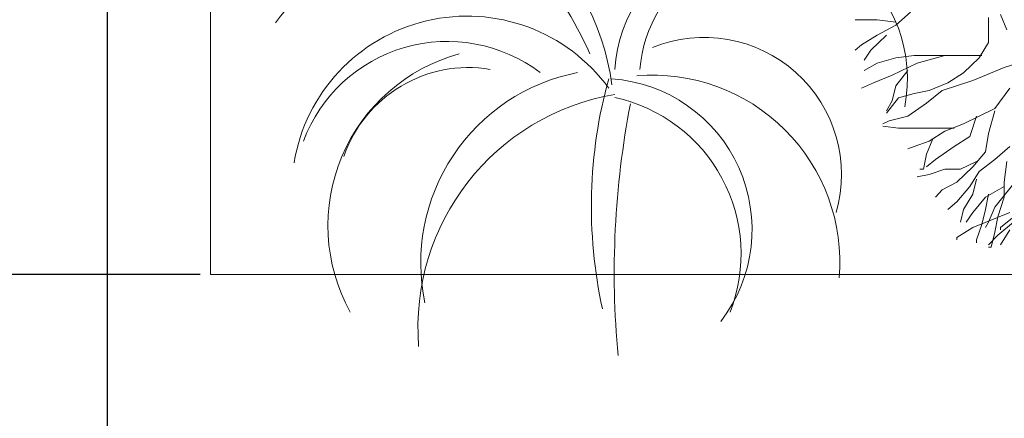
# Model space of a CAD drawing. Units: millimetres. Extents: x 595116 to 630915, y 909473 to 920225.
# Tile 11 of 134: x 629500 to 629559, y 919152 to 919176. Entities that reach past the tile are written whole.
import ezdxf

# ---------------------------------------------------------------- set-up
doc = ezdxf.new("R2010")
doc.units = ezdxf.units.MM
doc.layers.add('Dimension', color=3, linetype='Continuous', lineweight=18)
doc.layers.add('L-PLNT', color=85, linetype='Continuous', lineweight=13)
doc.styles.get("Standard").update_dxf_attribs({"font": 'arial.ttf'})
doc.dimstyles.new('ISO-25', dxfattribs={"dimtxt": 9, "dimasz": 6, "dimexe": 1.25, "dimexo": 0.625, "dimtad": 1, "dimlunit": 4, "dimtxsty": 'Standard', "dimcen": 2.5, "dimadec": 0, "dimazin": 0, "dimtfac": 1, "dimtmove": 0, "dimatfit": 3, "dimfxl": 1, "dimarcsym": 0})

# ---------------------------------------------------------------- blocks, each defined once
blk = doc.blocks.new('tree')
for centre, radius, start, end in [((629594.259, 919292.132), 6.965, 7.4001, 94.0059), ((629589.446, 919288.922), 12.167, 24.2477, 54.3726), ((629605.429, 919293.205), 4.185, 348.9977, 176.315), ((629605.915, 919293.144), 3.963, 69.3845, 175.231), ((629595.377, 919292.044), 4.722, 54.2484, 144.2167), ((629597.025, 919289.989), 5.01, 36.0581, 170.6542), ((629596.464, 919289.874), 4.4, 52.9074, 159.3471), ((629603.809, 919290.469), 3.92, 343.886, 112.2662), ((629598.153, 919288.998), 5.103, 105.3576, 208.8973), ((629597.068, 919289.758), 3.768, 80.4816, 161.0664), ((629601.247, 919287.941), 5.545, 101.0419, 191.8692), ((629602.329, 919287.957), 5.355, 355.2141, 94.8217), ((629614.329, 919289.554), 13.748, 164.5925, 192.323), ((629600.849, 919288.894), 4.324, 322.5461, 85.805), ((629602.391, 919286.088), 6.769, 99.681, 184.5451), ((629626.813, 919287.645), 25.579, 169.0753, 185.2889), ((629600.275, 919288.191), 4.585, 338.7925, 77.6921)]:
    blk.add_arc(centre, radius, start, end)
blk = doc.blocks.new('A$C143125F4')
for p, q in [((0.4158, 2.0204), (0.3282, 1.9443)), ((0.8753, 1.8412), (0.8753, 1.9891)), ((0.9464, 2.007), (0.9847, 1.9174)), ((0.2188, 1.9756), (0.0875, 1.9756)), ((0.3282, 1.9622), (0.2188, 1.9756)), ((0.3282, 1.9443), (0.2188, 1.886)), ((0.2188, 1.886), (0.1258, 1.8278)), ((0.2735, 1.886), (0.1805, 1.7964)), ((0.1258, 1.8278), (0.0875, 1.7964)), ((0.8206, 1.7516), (0.8753, 1.8412)), ((0.1805, 1.7964), (0.1422, 1.7382)), ((0.3282, 1.7516), (0.2188, 1.7203)), ((0.4376, 1.7651), (0.3282, 1.7516)), ((0.837, 1.7651), (0.4376, 1.7651)), ((0.6182, 1.7651), (0.4541, 1.7203)), ((0.7276, 1.662), (0.8206, 1.7516)), ((1.1488, 1.7516), (0.9683, 1.6934)), ((0.2188, 1.7203), (0.1422, 1.6755)), ((0.4541, 1.7203), (0.3063, 1.6486)), ((0.9683, 1.6934), (0.7823, 1.6172)), ((0.3063, 1.6486), (0.1969, 1.6038)), ((0.3993, 1.6755), (0.3282, 1.5859)), ((0.6346, 1.6038), (0.7276, 1.662)), ((0.1969, 1.6038), (0.1258, 1.5724)), ((0.3282, 1.5859), (0.3063, 1.4963)), ((0.5252, 1.559), (0.6346, 1.6038)), ((0.7823, 1.6172), (0.6018, 1.559)), ((1.0011, 1.5724), (0.9136, 1.4515)), ((0.2735, 1.4246), (0.3446, 1.5142)), ((0.3446, 1.5142), (0.4376, 1.5411)), ((0.4376, 1.5411), (0.5252, 1.559)), ((0.6018, 1.559), (0.5088, 1.4828)), ((0.3063, 1.4963), (0.2735, 1.438)), ((0.5088, 1.4828), (0.3993, 1.4067)), ((0.3993, 1.4067), (0.2899, 1.3798)), ((0.9136, 1.4515), (0.7276, 1.3619)), ((0.8042, 1.4067), (0.7659, 1.2857)), ((0.9136, 1.438), (0.8753, 1.3036)), ((0.2899, 1.3798), (0.2516, 1.3619)), ((0.3446, 1.335), (0.2516, 1.3484)), ((0.7276, 1.3619), (0.6182, 1.3171)), ((0.6729, 1.335), (0.3446, 1.335)), ((0.6182, 1.3171), (0.5252, 1.2588)), ((0.7659, 1.2857), (0.6729, 1.2275)), ((0.8753, 1.3036), (0.8589, 1.1961)), ((0.4376, 1.2275), (0.3993, 1.214)), ((0.5252, 1.2588), (0.4376, 1.2275)), ((0.5471, 1.2723), (0.5088, 1.1827)), ((0.6729, 1.2275), (0.5635, 1.1513)), ((1.0011, 1.2275), (0.9136, 1.1513)), ((0.5088, 1.1827), (0.4923, 1.0931)), ((0.8589, 1.1961), (0.7823, 1.1065)), ((0.5635, 1.1513), (0.5088, 1.1065)), ((0.7823, 1.1065), (0.6893, 1.0169)), ((0.8042, 1.1379), (0.7112, 1.0931)), ((0.9136, 1.1513), (0.8206, 1.0796)), ((0.9847, 1.1379), (0.9683, 1.0169)), ((0.5252, 1.0617), (0.4541, 1.0483)), ((0.4923, 1.0931), (0.4705, 1.0931)), ((0.6182, 1.0931), (0.5252, 1.0617)), ((0.7112, 1.0931), (0.6182, 1.0931)), ((0.8206, 1.0796), (0.7659, 0.99)), ((1.0558, 1.0483), (0.9136, 0.8691)), ((0.6893, 1.0169), (0.6018, 0.9721)), ((0.7659, 0.99), (0.6893, 0.9005)), ((0.8042, 1.0348), (0.7823, 0.9452)), ((0.9683, 0.99), (0.8589, 0.9273)), ((0.9683, 1.0169), (0.9683, 0.9273)), ((0.6018, 0.9721), (0.5635, 0.9273)), ((0.7823, 0.9452), (0.7276, 0.8557)), ((0.8753, 0.9452), (0.8589, 0.8557)), ((0.6893, 0.9005), (0.6346, 0.8557)), ((0.8589, 0.9273), (0.7823, 0.8377)), ((0.9683, 0.9273), (0.93, 0.8109)), ((1.1324, 0.9005), (0.9464, 0.7481)), ((0.7276, 0.8557), (0.7112, 0.7795)), ((0.7823, 0.8377), (0.744, 0.7795)), ((1.0011, 0.8377), (0.7823, 0.7481)), ((0.8589, 0.8557), (0.837, 0.7661)), ((0.9136, 0.8691), (0.8753, 0.7795)), ((0.837, 0.7661), (0.8042, 0.6765)), ((0.8753, 0.7795), (0.8589, 0.7481)), ((0.93, 0.8109), (0.9136, 0.7213)), ((1.023, 0.7795), (0.93, 0.7033)), ((0.7823, 0.7481), (0.6893, 0.6899)), ((0.93, 0.7033), (0.8753, 0.6451)), ((0.9136, 0.7213), (0.8917, 0.6317)), ((0.9464, 0.7481), (0.9464, 0.7347)), ((1.0011, 0.7347), (0.9464, 0.6451)), ((0.6893, 0.6899), (0.6893, 0.6765)), ((0.8042, 0.6765), (0.8042, 0.6585)), ((0.8917, 0.6317), (0.8753, 0.6317))]:
    blk.add_line(p, q)
blk = doc.blocks.new('*D215')
at = {"layer": 'Defpoints', "color": 0, "transparency": 16777216}
for p in [(629316.041, 919411.828), (629505.041, 919411.828), (629505.041, 918832.378)]:
    blk.add_point(p, dxfattribs=at)
at = {"layer": 'Dimension', "color": 0, "lineweight": -2, "transparency": 16777216}
for p, q in [((629316.041, 919411.203), (629316.041, 918831.128)), ((629505.041, 919411.203), (629505.041, 918831.128)), ((629322.041, 918832.378), (629499.041, 918832.378))]:
    blk.add_line(p, q, dxfattribs=at)
at = {"layer": 'Dimension', "color": 0, "transparency": 16777216}
for points in [[(629322.041, 918833.378), (629322.041, 918831.378), (629316.041, 918832.378)], [(629499.041, 918833.378), (629499.041, 918831.378), (629505.041, 918832.378)]]:
    blk.add_solid(points, dxfattribs=at)
at = {"layer": 'Dimension', "color": 0, "transparency": 16777216, "insert": (629410.541, 918837.598), "char_height": 9, "attachment_point": 5}
blk.add_mtext('15\'-9"', dxfattribs=at)
blk = doc.blocks.new('*D216')
at = {"layer": 'Defpoints', "color": 0, "transparency": 16777216}
for p in [(629505.041, 919411.828), (629743.541, 919411.928), (629743.541, 918832.378)]:
    blk.add_point(p, dxfattribs=at)
at = {"layer": 'Dimension', "color": 0, "lineweight": -2, "transparency": 16777216}
for p, q in [((629505.041, 919411.203), (629505.041, 918831.128)), ((629743.541, 919411.303), (629743.541, 918831.128)), ((629511.041, 918832.378), (629737.541, 918832.378))]:
    blk.add_line(p, q, dxfattribs=at)
at = {"layer": 'Dimension', "color": 0, "transparency": 16777216}
for points in [[(629511.041, 918833.378), (629511.041, 918831.378), (629505.041, 918832.378)], [(629737.541, 918833.378), (629737.541, 918831.378), (629743.541, 918832.378)]]:
    blk.add_solid(points, dxfattribs=at)
at = {"layer": 'Dimension', "color": 0, "transparency": 16777216, "insert": (629624.291, 918837.656), "char_height": 9, "attachment_point": 5}
blk.add_mtext('19\'-10 1/2"', dxfattribs=at)
blk = doc.blocks.new('*D221')
at = {"layer": 'Defpoints', "color": 0, "transparency": 16777216}
for p in [(629511.274, 919302.009), (629155.382, 919160.917), (629511.274, 919160.917)]:
    blk.add_point(p, dxfattribs=at)
at = {"layer": 'Dimension', "color": 0, "lineweight": -2, "transparency": 16777216}
for p, q in [((629510.649, 919302.009), (629154.132, 919302.009)), ((629155.382, 919296.009), (629155.382, 919166.917)), ((629510.649, 919160.917), (629154.132, 919160.917))]:
    blk.add_line(p, q, dxfattribs=at)
at = {"layer": 'Dimension', "color": 0, "transparency": 16777216}
for points in [[(629154.382, 919296.009), (629156.382, 919296.009), (629155.382, 919302.009)], [(629154.382, 919166.917), (629156.382, 919166.917), (629155.382, 919160.917)]]:
    blk.add_solid(points, dxfattribs=at)
at = {"layer": 'Dimension', "color": 0, "transparency": 16777216, "insert": (629150.162, 919231.463), "char_height": 9, "attachment_point": 5, "rotation": 90}
blk.add_mtext('11\'-9"', dxfattribs=at)

msp = doc.modelspace()

# ---------------------------------------------------------------- linework, layer by layer
at = {"layer": 'L-PLNT'}
for p, q in [((629511.274, 919302.009), (629511.274, 919160.917)), ((629511.274, 919160.917), (629824.951, 919160.917))]:
    msp.add_line(p, q, dxfattribs=at)

# ---------------------------------------------------------------- block references
for name, p, xscale, yscale, zscale in [('A$C143125F4', (629549.214, 919156.111), 10.20167662382051, 10.20167662382051, 10.20167662382051), ('tree', (-697468.256, -1018411.841), 2.107689410566463, 2.107689410566463, 2.107689410566463)]:
    msp.add_blockref(name, p, dxfattribs=dict(at, xscale=xscale, yscale=yscale, zscale=zscale))

# ---------------------------------------------------------------- dimensions: what is measured, and where the dimension line sits
at = {"layer": 'Dimension'}
for base, p1, p2, picture, middle in [((629505.041, 918832.378), (629316.041, 919411.828), (629505.041, 919411.828), '*D215', (629410.541, 918837.598)), ((629743.541, 918832.378), (629505.041, 919411.828), (629743.541, 919411.928), '*D216', (629624.291, 918837.656))]:
    dim = msp.add_linear_dim(base=base, p1=p1, p2=p2, dimstyle='ISO-25', override={"dimdec": 1, "dimlfac": 1, "dimrnd": 0, "dimzin": 1, "dimdsep": 46, "dimlunit": 4, "dimfrac": 2}, dxfattribs=at)
    dim.commit()
    dim.dimension.update_dxf_attribs({"geometry": picture, "text_midpoint": middle})
dim = msp.add_linear_dim(base=(629155.382, 919160.917), p1=(629511.274, 919302.009), p2=(629511.274, 919160.917), angle=90, dimstyle='ISO-25', override={"dimdec": 1, "dimlfac": 1, "dimrnd": 0, "dimzin": 1, "dimdsep": 46, "dimlunit": 4, "dimfrac": 2}, dxfattribs=at)
dim.commit()
dim.dimension.update_dxf_attribs({"geometry": '*D221', "text_midpoint": (629150.162, 919231.463)})

doc.saveas('drawing.dxf')
